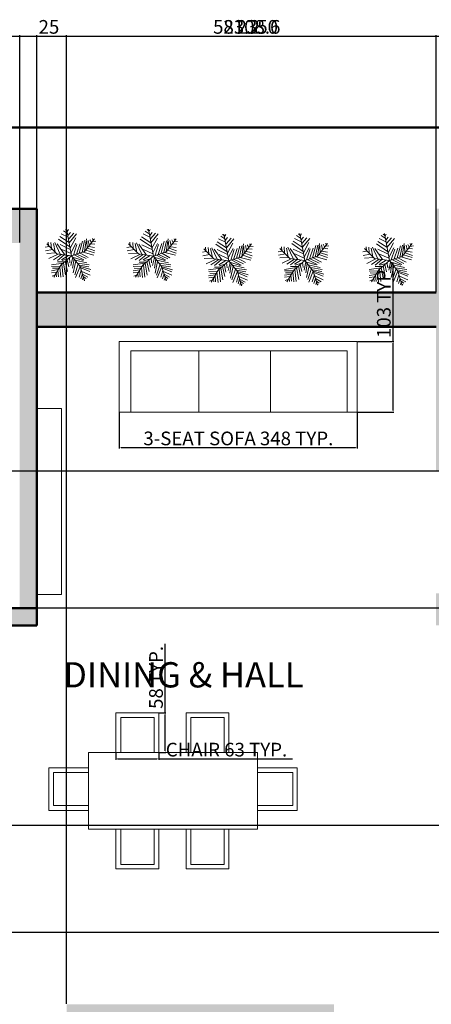
# Model space of a CAD drawing. Units: millimetres. Extents: x 1898 to 8115, y 727 to 4291.
# Tile 5 of 7: x 6177 to 6778, y 2277 to 3717. Entities that reach past the tile are written whole.
import ezdxf

# ---------------------------------------------------------------- set-up
doc = ezdxf.new("R2010")
doc.units = ezdxf.units.MM
for name, color, linetype, lineweight in [('A-ANNO-DIMS', 2, 'Continuous', 18), ('A-AREA-IDEN', 3, 'Continuous', 25), ('A-FURN', 8, 'Continuous', 18), ('A-WALL', 7, 'Continuous', 50), ('A-WALL-PATT', 8, 'Continuous', 13), ('L-PLNT', 112, 'Continuous', 18)]:
    doc.layers.add(name, color=color, linetype=linetype, lineweight=lineweight)
doc.styles.get("Standard").update_dxf_attribs({"font": 'arial.ttf'})
doc.dimstyles.new('ISO-25', dxfattribs={"dimtxt": 20, "dimasz": 2.5, "dimexe": 1.25, "dimexo": 0.625, "dimtad": 1, "dimtxsty": 'Standard', "dimcen": 2.5, "dimadec": 0, "dimazin": 0, "dimtfac": 1, "dimtmove": 0, "dimatfit": 3, "dimfxl": 1, "dimarcsym": 0})

# ---------------------------------------------------------------- blocks, each defined once
blk = doc.blocks.new('*U47')
for p, q in [((-7.288, 39.707), (-21.778, 46.673)), ((-8.737, 47.138), (-17.069, 52.711)), ((-10.186, 53.64), (-13.084, 55.962)), ((0, 0), (-10.5, 57)), ((-9.099, 51.782), (-6.563, 55.962)), ((-7.65, 43.423), (-2.578, 49.46)), ((-5.839, 35.992), (4.667, 48.067)), ((-5.114, 27.632), (10.463, 46.673)), ((-31.5, 4.5), (-52.5, 25.5)), ((-48.585, 21.131), (-49.309, 29.026)), ((-43.513, 28.561), (-42.427, 15.558)), ((-38.442, 26.239), (-34.819, 7.663)), ((-35.544, 28.097), (-24.314, 3.947)), ((-14.533, 2.09), (-30.834, 25.31)), ((-3.665, 19.273), (-27.574, 35.527)), ((-5.114, 28.097), (-24.676, 40.636)), ((-24.314, 23.917), (-2.941, 13.7)), ((-2.941, 16.486), (8.652, 37.85)), ((-1.129, 6.734), (9.014, 26.704)), ((3.942, 1.625), (11.187, 24.381)), ((10.101, 3.483), (17.708, 26.239)), ((16.259, 5.805), (23.142, 31.348)), ((22.055, 7.198), (27.489, 32.277)), ((27, 9), (48, 36)), ((27.127, 9.056), (31.112, 35.992)), ((31.836, 30.883), (32.561, 16.486)), ((35.096, 32.741), (37.27, 22.524)), ((38.719, 34.134), (41.979, 28.561)), ((40.53, 25.775), (48.862, 24.846)), ((43.791, 29.954), (51.036, 30.883)), ((44.153, 36.456), (45.239, 32.741)), ((-47.498, 19.737), (-55.83, 18.344)), ((-40.615, 13.7), (-55.105, 10.913)), ((-33.37, 6.269), (-52.207, 5.34)), ((-28.299, 3.483), (-47.86, -5.805)), ((-21.416, 3.018), (-38.079, -8.128)), ((0, 0), (-31.5, 4.5)), ((-15.982, 2.09), (-30.11, -9.521)), ((0, 0), (-22.5, -19.5)), ((-6.563, 1.161), (-21.416, -8.128)), ((-20.691, 13.7), (-1.129, 4.876)), ((0, 0), (27, 9)), ((0, 0), (18, -22.5)), ((6.478, 1.625), (26.04, -8.592)), ((11.187, 3.483), (30.749, -5.805)), ((18.07, 5.805), (35.096, -3.483)), ((24.229, 7.663), (46.688, 1.625)), ((29.662, 12.307), (48.137, 6.269)), ((33.285, 16.486), (48.862, 10.913)), ((36.183, 19.737), (48.137, 17.88)), ((-17.431, -15.094), (-42.789, -18.809)), ((-22.5, -19.5), (-37.5, -45)), ((-15.257, -12.772), (-30.11, -12.772)), ((-20.691, -18.345), (-17.793, -44.352)), ((-6.563, -5.805), (-19.967, -9.985)), ((-17.069, -15.094), (-12.721, -40.172)), ((-13.446, -11.378), (-8.737, -32.741)), ((-9.461, -8.592), (-6.201, -23.453)), ((-4.752, -3.483), (-3.665, -14.629)), ((2.493, -3.019), (-1.491, -20.202)), ((1.769, -2.555), (24.229, -9.521)), ((5.029, -6.27), (2.131, -25.775)), ((9.014, -11.378), (3.58, -35.992)), ((14.085, -16.951), (6.478, -40.172)), ((7.565, -9.056), (32.198, -14.629)), ((12.274, -15.094), (36.907, -18.809)), ((16.259, -19.738), (36.183, -22.989)), ((-28.299, -29.026), (-42.789, -31.348)), ((-24.314, -21.596), (-42.427, -22.06)), ((-30.834, -34.135), (-42.427, -35.528)), ((-34.457, -39.708), (-40.978, -42.494)), ((-26.849, -26.24), (-40.253, -25.775)), ((-32.646, -36.921), (-31.921, -44.352)), ((-29.023, -30.884), (-27.936, -43.887)), ((-25.038, -23.918), (-22.865, -45.281)), ((18.07, -22.524), (8.289, -45.745)), ((20.244, -30.419), (15.897, -44.816)), ((18, -22.5), (27, -52.5)), ((18.433, -22.524), (40.53, -29.026)), ((19.157, -25.311), (38.719, -33.206)), ((22.78, -37.85), (19.519, -48.532)), ((21.331, -32.741), (39.081, -40.636)), ((22.78, -38.314), (34.372, -44.816)), ((24.591, -45.745), (23.142, -50.854)), ((24.591, -43.423), (30.749, -47.603)), ((26.764, -49.925), (28.213, -50.854))]:
    blk.add_line(p, q)
blk = doc.blocks.new('SOFA-3SEAT')
for p, q in [((6339.2, 3143.3), (6339.2, 3232.9)), ((6339.2, 3232.9), (6655, 3232.9)), ((6438.4, 3232.9), (6438.4, 3143.3)), ((6543.3, 3232.9), (6543.3, 3143.3)), ((6655, 3232.9), (6655, 3143.3))]:
    blk.add_line(p, q)
blk.add_lwpolyline([(6322.2, 3246.6), (6669.9, 3246.6), (6669.9, 3143.3), (6322.2, 3143.3)], close=True)
blk = doc.blocks.new('CHAIR')
for p, q in [((6324.4, 2645.3), (6324.4, 2696.7)), ((6324.4, 2696.7), (6373, 2696.7)), ((6373, 2696.7), (6373, 2645.3))]:
    blk.add_line(p, q)
blk.add_lwpolyline([(6317.3, 2645.3), (6379.8, 2645.3), (6379.8, 2703.3), (6317.3, 2703.3)], close=True)
blk = doc.blocks.new('*D51')
at = {"layer": 'A-ANNO-DIMS', "color": 0, "lineweight": -2, "transparency": 16777216}
for p, q in [((6317.3, 2644.7), (6317.3, 2634.7)), ((6319.8, 2636), (6377.3, 2636)), ((6379.8, 2644.7), (6379.8, 2634.7)), ((6379.8, 2636), (6575.4, 2636))]:
    blk.add_line(p, q, dxfattribs=at)
at = {"layer": 'A-ANNO-DIMS', "color": 0, "transparency": 16777216}
for points in [[(6319.8, 2636.4), (6319.8, 2635.5), (6317.3, 2636)], [(6377.3, 2636.4), (6377.3, 2635.5), (6379.8, 2636)]]:
    blk.add_solid(points, dxfattribs=at)
at = {"layer": 'Defpoints', "color": 0, "transparency": 16777216}
for p in [(6317.3, 2645.3), (6379.8, 2645.3), (6379.8, 2636)]:
    blk.add_point(p, dxfattribs=at)
at = {"layer": 'A-ANNO-DIMS', "color": 0, "transparency": 16777216, "insert": (6478.8, 2646.9), "char_height": 20, "attachment_point": 5}
blk.add_mtext('CHAIR 63 TYP.', dxfattribs=at)
blk = doc.blocks.new('*D52')
at = {"layer": 'A-ANNO-DIMS', "color": 0, "lineweight": -2, "transparency": 16777216}
for p, q in [((6389.2, 2703.3), (6389.2, 2804.4)), ((6380.4, 2703.3), (6390.4, 2703.3)), ((6389.2, 2647.8), (6389.2, 2700.8)), ((6380.4, 2645.3), (6390.4, 2645.3))]:
    blk.add_line(p, q, dxfattribs=at)
at = {"layer": 'A-ANNO-DIMS', "color": 0, "transparency": 16777216}
for points in [[(6388.8, 2700.8), (6389.6, 2700.8), (6389.2, 2703.3)], [(6388.8, 2647.8), (6389.6, 2647.8), (6389.2, 2645.3)]]:
    blk.add_solid(points, dxfattribs=at)
at = {"layer": 'Defpoints', "color": 0, "transparency": 16777216}
for p in [(6379.8, 2703.3), (6389.2, 2703.3), (6379.8, 2645.3)]:
    blk.add_point(p, dxfattribs=at)
at = {"layer": 'A-ANNO-DIMS', "color": 0, "transparency": 16777216, "insert": (6378.4, 2755.1), "char_height": 20, "attachment_point": 5, "rotation": 90}
blk.add_mtext('58 TYP.', dxfattribs=at)
blk = doc.blocks.new('*D55')
at = {"layer": 'A-ANNO-DIMS', "color": 0, "lineweight": -2, "transparency": 16777216}
for p, q in [((6322.2, 3142.7), (6322.2, 3089.9)), ((6669.9, 3142.7), (6669.9, 3089.9)), ((6324.7, 3091.2), (6667.4, 3091.2))]:
    blk.add_line(p, q, dxfattribs=at)
at = {"layer": 'A-ANNO-DIMS', "color": 0, "transparency": 16777216}
for points in [[(6324.7, 3091.6), (6324.7, 3090.7), (6322.2, 3091.2)], [(6667.4, 3091.6), (6667.4, 3090.7), (6669.9, 3091.2)]]:
    blk.add_solid(points, dxfattribs=at)
at = {"layer": 'Defpoints', "color": 0, "transparency": 16777216}
for p in [(6322.2, 3143.3), (6669.9, 3143.3), (6669.9, 3091.2)]:
    blk.add_point(p, dxfattribs=at)
at = {"layer": 'A-ANNO-DIMS', "color": 0, "transparency": 16777216, "insert": (6496.1, 3102.1), "char_height": 20, "attachment_point": 5}
blk.add_mtext('3-SEAT SOFA 348 TYP.', dxfattribs=at)
blk = doc.blocks.new('*D56')
at = {"layer": 'A-ANNO-DIMS', "color": 0, "lineweight": -2, "transparency": 16777216}
for p, q in [((6722.1, 3246.6), (6722.1, 3361.3)), ((6670.5, 3246.6), (6723.3, 3246.6)), ((6722.1, 3145.8), (6722.1, 3244.1)), ((6670.5, 3143.3), (6723.3, 3143.3))]:
    blk.add_line(p, q, dxfattribs=at)
at = {"layer": 'A-ANNO-DIMS', "color": 0, "transparency": 16777216}
for points in [[(6721.7, 3244.1), (6722.5, 3244.1), (6722.1, 3246.6)], [(6721.7, 3145.8), (6722.5, 3145.8), (6722.1, 3143.3)]]:
    blk.add_solid(points, dxfattribs=at)
at = {"layer": 'Defpoints', "color": 0, "transparency": 16777216}
for p in [(6669.9, 3246.6), (6722.1, 3246.6), (6669.9, 3143.3)]:
    blk.add_point(p, dxfattribs=at)
at = {"layer": 'A-ANNO-DIMS', "color": 0, "transparency": 16777216, "insert": (6711.2, 3305.2), "char_height": 20, "attachment_point": 5, "rotation": 90}
blk.add_mtext('103 TYP.', dxfattribs=at)
blk = doc.blocks.new('*D57')
at = {"layer": 'A-ANNO-DIMS', "color": 0, "lineweight": -2, "transparency": 16777216}
for p, q in [((5348.6, 3560.4), (5348.6, 3694.5)), ((5351.1, 3693.2), (7696.3, 3693.2)), ((7698.8, 3560.4), (7698.8, 3694.5))]:
    blk.add_line(p, q, dxfattribs=at)
at = {"layer": 'A-ANNO-DIMS', "color": 0, "transparency": 16777216}
for points in [[(5351.1, 3693.7), (5351.1, 3692.8), (5348.6, 3693.2)], [(7696.3, 3693.7), (7696.3, 3692.8), (7698.8, 3693.2)]]:
    blk.add_solid(points, dxfattribs=at)
at = {"layer": 'Defpoints', "color": 0, "transparency": 16777216}
for p in [(7698.8, 3693.2), (5348.6, 3559.7), (7698.8, 3559.7)]:
    blk.add_point(p, dxfattribs=at)
at = {"layer": 'A-ANNO-DIMS', "color": 0, "transparency": 16777216, "insert": (6523.7, 3704.1), "char_height": 20, "attachment_point": 5}
blk.add_mtext('2350', dxfattribs=at)
blk = doc.blocks.new('*D58')
at = {"layer": 'A-ANNO-DIMS', "color": 0, "lineweight": -2, "transparency": 16777216}
for p, q in [((5461.6, 3441.3), (5461.6, 3694.5)), ((5464.1, 3693.2), (7567.7, 3693.2)), ((7570.2, 3441.3), (7570.2, 3694.5))]:
    blk.add_line(p, q, dxfattribs=at)
at = {"layer": 'A-ANNO-DIMS', "color": 0, "transparency": 16777216}
for points in [[(5464.1, 3693.7), (5464.1, 3692.8), (5461.6, 3693.2)], [(7567.7, 3693.7), (7567.7, 3692.8), (7570.2, 3693.2)]]:
    blk.add_solid(points, dxfattribs=at)
at = {"layer": 'Defpoints', "color": 0, "transparency": 16777216}
for p in [(7570.2, 3693.2), (5461.6, 3440.7), (7570.2, 3440.7)]:
    blk.add_point(p, dxfattribs=at)
at = {"layer": 'A-ANNO-DIMS', "color": 0, "transparency": 16777216, "insert": (6515.9, 3704.1), "char_height": 20, "attachment_point": 5}
blk.add_mtext('2108.6', dxfattribs=at)
blk = doc.blocks.new('*D64')
at = {"layer": 'A-ANNO-DIMS', "color": 0, "lineweight": -2, "transparency": 16777216}
for p, q in [((5511.6, 3391.3), (5511.6, 3694.5)), ((5514.1, 3693.2), (6174.2, 3693.2)), ((6176.7, 3391.3), (6176.7, 3694.5))]:
    blk.add_line(p, q, dxfattribs=at)
at = {"layer": 'A-ANNO-DIMS', "color": 0, "transparency": 16777216}
for points in [[(5514.1, 3693.7), (5514.1, 3692.8), (5511.6, 3693.2)], [(6174.2, 3693.7), (6174.2, 3692.8), (6176.7, 3693.2)]]:
    blk.add_solid(points, dxfattribs=at)
at = {"layer": 'Defpoints', "color": 0, "transparency": 16777216}
for p in [(6176.7, 3693.2), (5511.6, 3390.7), (6176.7, 3390.7)]:
    blk.add_point(p, dxfattribs=at)
at = {"layer": 'A-ANNO-DIMS', "color": 0, "transparency": 16777216, "insert": (5844.2, 3704.1), "char_height": 20, "attachment_point": 5}
blk.add_mtext('665.1', dxfattribs=at)
blk = doc.blocks.new('*D65')
at = {"layer": 'A-ANNO-DIMS', "color": 0, "lineweight": -2, "transparency": 16777216}
for p, q in [((6176.7, 3391.3), (6176.7, 3694.5)), ((6179.2, 3693.2), (6199.2, 3693.2)), ((6201.7, 3318.6), (6201.7, 3694.5)), ((6201.7, 3693.2), (6234.6, 3693.2))]:
    blk.add_line(p, q, dxfattribs=at)
at = {"layer": 'A-ANNO-DIMS', "color": 0, "transparency": 16777216}
for points in [[(6179.2, 3693.7), (6179.2, 3692.8), (6176.7, 3693.2)], [(6199.2, 3693.7), (6199.2, 3692.8), (6201.7, 3693.2)]]:
    blk.add_solid(points, dxfattribs=at)
at = {"layer": 'Defpoints', "color": 0, "transparency": 16777216}
for p in [(6201.7, 3693.2), (6176.7, 3390.7), (6201.7, 3318)]:
    blk.add_point(p, dxfattribs=at)
at = {"layer": 'A-ANNO-DIMS', "color": 0, "transparency": 16777216, "insert": (6219.4, 3704.1), "char_height": 20, "attachment_point": 5}
blk.add_mtext('25', dxfattribs=at)
blk = doc.blocks.new('*D66')
at = {"layer": 'A-ANNO-DIMS', "color": 0, "lineweight": -2, "transparency": 16777216}
for p, q in [((6201.7, 3318.6), (6201.7, 3694.5)), ((6204.2, 3693.2), (6782.4, 3693.2)), ((6784.9, 3318.6), (6784.9, 3694.5))]:
    blk.add_line(p, q, dxfattribs=at)
at = {"layer": 'A-ANNO-DIMS', "color": 0, "transparency": 16777216}
for points in [[(6204.2, 3693.7), (6204.2, 3692.8), (6201.7, 3693.2)], [(6782.4, 3693.7), (6782.4, 3692.8), (6784.9, 3693.2)]]:
    blk.add_solid(points, dxfattribs=at)
at = {"layer": 'Defpoints', "color": 0, "transparency": 16777216}
for p in [(6784.9, 3693.2), (6201.7, 3318), (6784.9, 3318)]:
    blk.add_point(p, dxfattribs=at)
at = {"layer": 'A-ANNO-DIMS', "color": 0, "transparency": 16777216, "insert": (6493.3, 3704.1), "char_height": 20, "attachment_point": 5}
blk.add_mtext('583.2', dxfattribs=at)
blk = doc.blocks.new('*D106')
at = {"layer": 'A-ANNO-DIMS', "color": 0, "lineweight": -2, "transparency": 16777216}
for p, q in [((5989.6, 2277.6), (5989.6, 3694.5)), ((5992.1, 3693.2), (6242.8, 3693.2)), ((6245.3, 2277.6), (6245.3, 3694.5))]:
    blk.add_line(p, q, dxfattribs=at)
at = {"layer": 'A-ANNO-DIMS', "color": 0, "transparency": 16777216}
for points in [[(5992.1, 3693.7), (5992.1, 3692.8), (5989.6, 3693.2)], [(6242.8, 3693.7), (6242.8, 3692.8), (6245.3, 3693.2)]]:
    blk.add_solid(points, dxfattribs=at)
at = {"layer": 'Defpoints', "color": 0, "transparency": 16777216}
for p in [(6245.3, 3693.2), (5989.6, 2277), (6245.3, 2277)]:
    blk.add_point(p, dxfattribs=at)
at = {"layer": 'A-ANNO-DIMS', "color": 0, "transparency": 16777216, "insert": (6117.4, 3704.1), "char_height": 20, "attachment_point": 5}
blk.add_mtext('255.7', dxfattribs=at)
blk = doc.blocks.new('*D110')
at = {"layer": 'A-ANNO-DIMS', "color": 0, "lineweight": -2, "transparency": 16777216}
for p, q in [((6809.3, 3057), (5213.8, 3057)), ((5215.1, 2858.8), (5215.1, 3054.5)), ((6809.3, 2856.3), (5213.8, 2856.3))]:
    blk.add_line(p, q, dxfattribs=at)
at = {"layer": 'A-ANNO-DIMS', "color": 0, "transparency": 16777216}
for points in [[(5214.6, 3054.5), (5215.5, 3054.5), (5215.1, 3057)], [(5214.6, 2858.8), (5215.5, 2858.8), (5215.1, 2856.3)]]:
    blk.add_solid(points, dxfattribs=at)
at = {"layer": 'Defpoints', "color": 0, "transparency": 16777216}
for p in [(5215.1, 3057), (6809.9, 3057), (6809.9, 2856.3)]:
    blk.add_point(p, dxfattribs=at)
at = {"layer": 'A-ANNO-DIMS', "color": 0, "transparency": 16777216, "insert": (5204.2, 2956.6), "char_height": 20, "attachment_point": 5, "rotation": 90}
blk.add_mtext('200.72', dxfattribs=at)
blk = doc.blocks.new('*D113')
at = {"layer": 'A-ANNO-DIMS', "color": 0, "lineweight": -2, "transparency": 16777216}
for p, q in [((6965.2, 2538.5), (5213.8, 2538.5)), ((5215.1, 2536), (5215.1, 2384.6)), ((6965.2, 2382.1), (5213.8, 2382.1))]:
    blk.add_line(p, q, dxfattribs=at)
at = {"layer": 'A-ANNO-DIMS', "color": 0, "transparency": 16777216}
for points in [[(5214.6, 2536), (5215.5, 2536), (5215.1, 2538.5)], [(5214.6, 2384.6), (5215.5, 2384.6), (5215.1, 2382.1)]]:
    blk.add_solid(points, dxfattribs=at)
at = {"layer": 'Defpoints', "color": 0, "transparency": 16777216}
for p in [(6965.8, 2538.5), (5215.1, 2382.1), (6965.8, 2382.1)]:
    blk.add_point(p, dxfattribs=at)
at = {"layer": 'A-ANNO-DIMS', "color": 0, "transparency": 16777216, "insert": (5204.2, 2460.3), "char_height": 20, "attachment_point": 5, "rotation": 90}
blk.add_mtext('156.42', dxfattribs=at)

msp = doc.modelspace()

# ---------------------------------------------------------------- hatches: boundary and pattern name
at = {"layer": 'A-WALL-PATT'}
h = msp.add_hatch(color=256, dxfattribs=at)
h.dxf.hatch_style = 1
h.paths.add_polyline_path([(6201.726, 3440.661), (5461.585, 3440.661), (5461.585, 3265.221), (5511.585, 3265.221), (5511.585, 3390.661), (6176.726, 3390.661), (6176.726, 2856.284), (6201.726, 2856.284)])
h.paths.add_polyline_path([(6784.895, 3318.017), (6201.726, 3318.017), (6201.726, 3268.017), (6784.895, 3268.017)])
h.paths.add_polyline_path([(7570.217, 3440.661), (6784.895, 3440.661), (6784.895, 3057.009), (6809.895, 3057.009), (6809.895, 3390.661), (7520.217, 3390.661), (7520.217, 3300.311), (7570.217, 3300.311)])
h.paths.add_polyline_path([(7570.217, 3000.359), (7520.217, 3000.359), (7520.217, 2758.681), (7570.217, 2758.681)])
h.paths.add_polyline_path([(7520.217, 2856.284), (7194.283, 2856.284), (6784.895, 2856.284), (6784.895, 2831.284), (7520.217, 2831.284)])
h.paths.add_polyline_path([(6809.895, 2878.069), (6784.895, 2878.069), (6784.895, 2856.284), (6809.895, 2856.284)])
h.paths.add_polyline_path([(6201.726, 2856.284), (6176.726, 2856.284), (6161.551, 2856.284), (6161.551, 2831.284), (6201.726, 2831.284)])
h.paths.add_polyline_path([(5905.861, 2856.284), (5511.585, 2856.284), (5511.585, 2831.284), (5905.861, 2831.284)])
h.paths.add_polyline_path([(5511.585, 2965.269), (5461.585, 2965.269), (5461.585, 2698.678), (5511.585, 2698.678)])
h.paths.add_polyline_path([(5511.585, 2398.725), (5461.585, 2398.725), (5461.585, 2088.028), (5511.585, 2088.028)])
h.paths.add_polyline_path([(5989.6, 2238.621), (5989.6, 2276.975), (5511.585, 2276.975), (5511.585, 2226.975), (5989.865, 2226.975, -0.01139164)])
h.paths.add_polyline_path([(6636.013, 2276.975), (6245.29, 2276.975), (6245.29, 2238.621), (6245.29, 2226.975), (6636.013, 2226.975), (6636.013, 2238.621)])
h.paths.add_polyline_path([(7570.217, 2359.481), (7520.217, 2359.481), (7520.217, 2326.802), (7520.217, 2276.975), (6891.704, 2276.975), (6891.704, 2238.621, -0.01139164), (6891.439, 2226.975), (7570.217, 2226.975)])
h.paths.add_polyline_path([(7145.586, 2531.644), (6989.313, 2531.644), (6989.313, 2538.488), (7145.735, 2538.488), (7145.735, 2531.644), (7145.586, 2531.644, -0.39860379), (6990.849, 2382.073), (6990.849, 2276.975), (6965.849, 2276.975), (6965.849, 2382.065), (6989.313, 2382.065, 0.40145271)])
h.paths.add_polyline_path([(6990.849, 2596.561), (6989.313, 2596.561), (6965.849, 2596.561), (6965.849, 2538.488), (6990.849, 2538.488)])
h.paths.add_polyline_path([(6990.849, 2831.284), (6965.849, 2831.284), (6965.849, 2752.984), (6990.849, 2752.984)])
h.paths.add_polyline_path([(7570.217, 2638.517), (7520.217, 2638.517), (7520.217, 2625.002), (7520.217, 2479.644), (7570.217, 2479.644)])
h.paths.add_polyline_path([(7520.217, 2579.13), (6990.849, 2579.13), (6990.849, 2554.13), (7520.217, 2554.13)])

# ---------------------------------------------------------------- linework, layer by layer
at = {"layer": 'A-FURN'}
for points in [[(6201.726, 3148.473), (6237.937, 3148.473), (6237.937, 2876.649), (6201.726, 2876.649)], [(6277.28, 2645.342), (6524.124, 2645.342), (6524.124, 2532.981), (6277.28, 2532.981)]]:
    msp.add_lwpolyline(points, close=True, dxfattribs=at)
at = {"layer": 'A-WALL'}
for p, q in [((5461.585, 3440.661), (6201.726, 3440.661)), ((6201.726, 3440.661), (6201.726, 2856.284)), ((6201.726, 3318.017), (6784.895, 3318.017)), ((6201.726, 3268.017), (6784.895, 3268.017)), ((6161.551, 2856.284), (6201.726, 2856.284)), ((6201.726, 2856.284), (6201.726, 2831.284)), ((6161.551, 2831.284), (6201.726, 2831.284))]:
    msp.add_line(p, q, dxfattribs=at)
msp.add_lwpolyline([(5348.551, 3559.737), (7698.767, 3559.737), (7698.767, 1496.544), (5348.551, 1496.544)], close=True, dxfattribs=at)

# ---------------------------------------------------------------- block references
at = {"layer": 'A-FURN'}
for name, p in [('SOFA-3SEAT', (0, 0)), ('CHAIR', (0, 0)), ('CHAIR', (102.334, 0))]:
    msp.add_blockref(name, p, dxfattribs=at)
at = {"layer": 'A-FURN', "rotation": 90.00000000000038}
msp.add_blockref('CHAIR', (8922.622, -3756.726), dxfattribs=at)
at = {"layer": 'A-FURN', "extrusion": (0, 0, -1), "zscale": -1}
for p, rotation in [((-3878.782, -3756.726), 90.00000000000036), ((0, 5178.323), 180), ((-102.334, 5178.323), 180)]:
    msp.add_blockref('CHAIR', p, dxfattribs=dict(at, rotation=rotation))
at = {"layer": 'L-PLNT', "xscale": 0.6924237731587986, "yscale": 0.6924237731587986, "zscale": 0.6924237731587986}
for p in [(6252.547, 3371.699), (6371.95, 3371.517), (6482.214, 3364.261), (6593.088, 3365.003), (6716.756, 3364.822)]:
    msp.add_blockref('*U47', p, dxfattribs=at)

# ---------------------------------------------------------------- texts
at = {"layer": 'A-AREA-IDEN', "insert": (6240.212, 2777.428), "char_height": 36.98144, "attachment_point": 1}
msp.add_mtext_dynamic_manual_height_columns('DINING & HALL', width=5503.90807, gutter_width=184.907, heights=[0], dxfattribs=at)

# ---------------------------------------------------------------- dimensions: what is measured, and where the dimension line sits
at = {"layer": 'A-ANNO-DIMS'}
for base, p1, p2, override, picture, middle in [((7698.767, 3693.237), (5348.551, 3559.737), (7698.767, 3559.737), {"dimdec": 0, "dimlfac": 1, "dimrnd": 0, "dimzin": 0, "dimdsep": 46, "dimlunit": 2}, '*D57', (6523.659, 3704.08)), ((7570.217, 3693.237), (5461.585, 3440.661), (7570.217, 3440.661), {"dimdec": 1, "dimlfac": 1, "dimrnd": 0, "dimzin": 0, "dimdsep": 46, "dimlunit": 2}, '*D58', (6515.901, 3704.073)), ((6176.726, 3693.237), (5511.585, 3390.661), (6176.726, 3390.661), {"dimdec": 1, "dimlfac": 1, "dimrnd": 0, "dimzin": 0, "dimdsep": 46, "dimlunit": 2}, '*D64', (5844.155, 3704.073)), ((6245.29, 3693.237), (5989.6, 2276.975), (6245.29, 2276.975), {"dimdec": 1, "dimlfac": 1, "dimrnd": 0, "dimzin": 0, "dimdsep": 46, "dimlunit": 2}, '*D106', (6117.445, 3704.073)), ((6201.726, 3693.237), (6176.726, 3390.661), (6201.726, 3318.017), {"dimdec": 0, "dimlfac": 1, "dimrnd": 0, "dimzin": 0, "dimdsep": 46, "dimlunit": 2}, '*D65', (6219.421, 3704.073)), ((6784.895, 3693.237), (6201.726, 3318.017), (6784.895, 3318.017), {"dimdec": 1, "dimlfac": 1, "dimrnd": 0, "dimzin": 0, "dimdsep": 46, "dimlunit": 2}, '*D66', (6493.31, 3704.08))]:
    dim = msp.add_linear_dim(base=base, p1=p1, p2=p2, dimstyle='ISO-25', override=override, dxfattribs=at)
    dim.commit()
    dim.dimension.update_dxf_attribs({"geometry": picture, "text_midpoint": middle})
for base, p1, p2, picture, middle in [((6722.082, 3246.585), (6669.923, 3143.32), (6669.923, 3246.585), '*D56', (6711.238, 3305.214)), ((6389.192, 2703.28), (6379.816, 2645.342), (6379.816, 2703.28), '*D52', (6378.356, 2755.082))]:
    dim = msp.add_linear_dim(base=base, p1=p1, p2=p2, angle=90, text='<> TYP.', dimstyle='ISO-25', override={"dimdec": 0, "dimrnd": 0, "dimzin": 0, "dimlunit": 2}, dxfattribs=at)
    dim.commit()
    dim.dimension.update_dxf_attribs({"geometry": picture, "text_midpoint": middle})
for base, p1, p2, text, picture, middle in [((6669.923, 3091.161), (6322.201, 3143.32), (6669.923, 3143.32), '3-SEAT SOFA <> TYP.', '*D55', (6496.062, 3102.141)), ((6379.816, 2635.966), (6317.311, 2645.342), (6379.816, 2645.342), 'CHAIR <> TYP.', '*D51', (6478.849, 2646.939))]:
    dim = msp.add_linear_dim(base=base, p1=p1, p2=p2, text=text, dimstyle='ISO-25', override={"dimdec": 0, "dimrnd": 0, "dimzin": 0, "dimlunit": 2}, dxfattribs=at)
    dim.commit()
    dim.dimension.update_dxf_attribs({"geometry": picture, "text_midpoint": middle})
for base, p1, p2, picture, middle in [((5215.0506, 3057.0088), (6809.8949, 2856.2845), (6809.8949, 3057.0088), '*D110', (5204.2141, 2956.6467)), ((5215.051, 2382.065), (6965.849, 2538.488), (6965.849, 2382.065), '*D113', (5204.214, 2460.277))]:
    dim = msp.add_linear_dim(base=base, p1=p1, p2=p2, angle=90, dimstyle='ISO-25', override={"dimdec": 2, "dimlfac": 1, "dimrnd": 0, "dimzin": 0, "dimdsep": 46, "dimlunit": 2}, dxfattribs=at)
    dim.commit()
    dim.dimension.update_dxf_attribs({"geometry": picture, "text_midpoint": middle})

doc.saveas('drawing.dxf')
